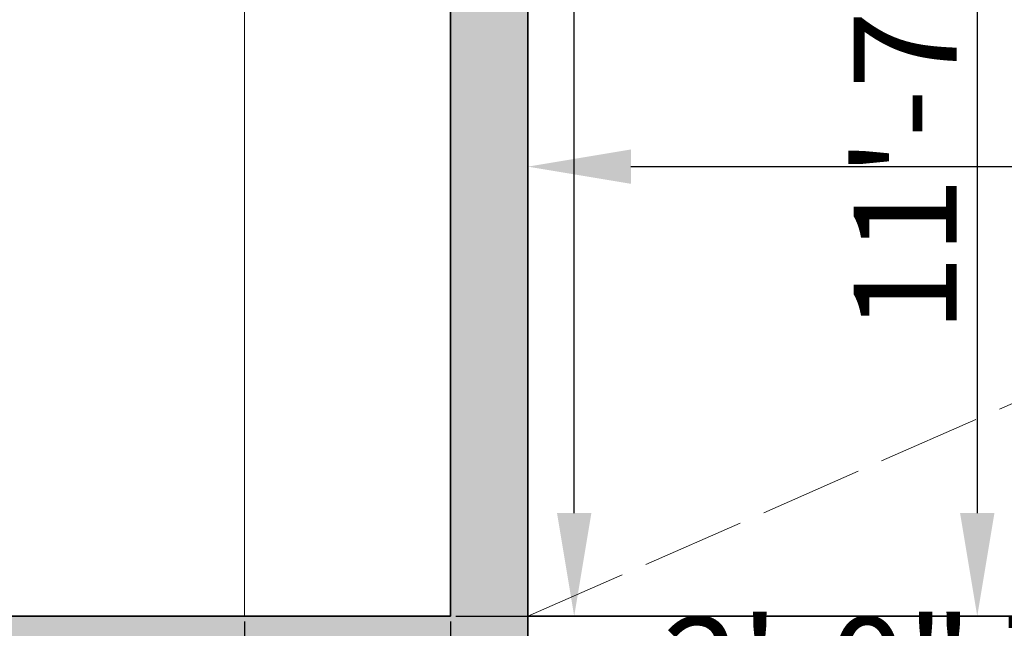
# Model space of a CAD drawing. Units: inches. Extents: x 2083 to 3317, y 1141 to 2115.
# Tile 86 of 256: x 2486 to 2600, y 1271 to 1342. Entities that reach past the tile are written whole.
import ezdxf

# ---------------------------------------------------------------- set-up
doc = ezdxf.new("R2010")
doc.units = ezdxf.units.IN
doc.linetypes.add('ACAD_ISO02W100', pattern=[15, 12, -3])
for name, color, linetype, lineweight in [('A-ANNO-DIMS', 2, 'Continuous', 18), ('A-FLOR-CASE', 8, 'Continuous', 18), ('A-FLOR-OPEN', 8, 'ACAD_ISO02W100', 13), ('A-WALL', 7, 'Continuous', 35)]:
    doc.layers.add(name, color=color, linetype=linetype, lineweight=lineweight)
doc.layers.add('A-WALL-PATT', color=251, linetype='Continuous', lineweight=13, true_color=0x636466)
doc.styles.get("Standard").update_dxf_attribs({"font": 'arial.ttf'})
doc.dimstyles.new('ISO-25', dxfattribs={"dimtxt": 12, "dimasz": 12, "dimexe": 1.25, "dimexo": 0.625, "dimtad": 1, "dimlunit": 3, "dimtxsty": 'Standard', "dimcen": 2.5, "dimadec": 0, "dimazin": 0, "dimtfac": 1, "dimtmove": 0, "dimatfit": 3, "dimfxl": 1, "dimarcsym": 0})

# ---------------------------------------------------------------- blocks, each defined once
blk = doc.blocks.new('CASEWORK-96X24')
for q in [(0, 0), (24, 96)]:
    blk.add_line((0, 96), q)
blk = doc.blocks.new('*D24')
at = {"layer": 'A-ANNO-DIMS', "color": 0, "lineweight": -2, "transparency": 16777216}
for p, q in [((2550.36, 1368.26), (2550.36, 1556.98)), ((2536.58, 1368.26), (2551.61, 1368.26)), ((2550.36, 1284.26), (2550.36, 1356.26)), ((2536.58, 1272.26), (2551.61, 1272.26))]:
    blk.add_line(p, q, dxfattribs=at)
at = {"layer": 'A-ANNO-DIMS', "color": 0, "transparency": 16777216}
for points in [[(2548.36, 1356.26), (2552.36, 1356.26), (2550.36, 1368.26)], [(2548.36, 1284.26), (2552.36, 1284.26), (2550.36, 1272.26)]]:
    blk.add_solid(points, dxfattribs=at)
at = {"layer": 'Defpoints', "color": 0, "transparency": 16777216}
for p in [(2535.96, 1368.26), (2550.36, 1368.26), (2535.96, 1272.26)]:
    blk.add_point(p, dxfattribs=at)
at = {"layer": 'A-ANNO-DIMS', "color": 0, "transparency": 16777216, "insert": (2543.53, 1468.62), "char_height": 12, "attachment_point": 5, "rotation": 90}
blk.add_mtext('CASEWORK 8\'-0" TYP.', dxfattribs=at)
blk = doc.blocks.new('*D25')
at = {"layer": 'A-ANNO-DIMS', "color": 0, "lineweight": -2, "transparency": 16777216}
for p, q in [((2511.96, 1271.64), (2511.96, 1256.61)), ((2535.96, 1271.64), (2535.96, 1256.61)), ((2499.96, 1257.86), (2487.96, 1257.86)), ((2511.96, 1257.86), (2535.96, 1257.86)), ((2547.96, 1257.86), (2634.56, 1257.86))]:
    blk.add_line(p, q, dxfattribs=at)
at = {"layer": 'A-ANNO-DIMS', "color": 0, "transparency": 16777216}
for points in [[(2499.96, 1259.86), (2499.96, 1255.86), (2511.96, 1257.86)], [(2547.96, 1259.86), (2547.96, 1255.86), (2535.96, 1257.86)]]:
    blk.add_solid(points, dxfattribs=at)
at = {"layer": 'Defpoints', "color": 0, "transparency": 16777216}
for p in [(2511.96, 1272.26), (2535.96, 1272.26), (2535.96, 1257.86)]:
    blk.add_point(p, dxfattribs=at)
at = {"layer": 'A-ANNO-DIMS', "color": 0, "transparency": 16777216, "insert": (2597.26, 1264.61), "char_height": 12, "attachment_point": 5}
blk.add_mtext('2\'-0" TYP.', dxfattribs=at)
blk = doc.blocks.new('*D66')
at = {"layer": 'A-ANNO-DIMS', "color": 0, "lineweight": -2, "transparency": 16777216}
for p, q in [((2544.96, 1272.89), (2544.96, 1325.86)), ((2862.96, 1272.89), (2862.96, 1325.86)), ((2556.96, 1324.61), (2850.96, 1324.61))]:
    blk.add_line(p, q, dxfattribs=at)
at = {"layer": 'A-ANNO-DIMS', "color": 0, "transparency": 16777216}
for points in [[(2556.96, 1326.61), (2556.96, 1322.61), (2544.96, 1324.61)], [(2850.96, 1326.61), (2850.96, 1322.61), (2862.96, 1324.61)]]:
    blk.add_solid(points, dxfattribs=at)
at = {"layer": 'Defpoints', "color": 0, "transparency": 16777216}
for p in [(2862.96, 1324.61), (2544.96, 1272.26), (2862.96, 1272.26)]:
    blk.add_point(p, dxfattribs=at)
at = {"layer": 'A-ANNO-DIMS', "color": 0, "transparency": 16777216, "insert": (2703.96, 1331.36), "char_height": 12, "attachment_point": 5}
blk.add_mtext('26\'-6"', dxfattribs=at)
blk = doc.blocks.new('*D67')
at = {"layer": 'A-ANNO-DIMS', "color": 0, "lineweight": -2, "transparency": 16777216}
for p, q in [((2545.58, 1411.76), (2598.56, 1411.76)), ((2597.31, 1399.76), (2597.31, 1284.26)), ((2545.58, 1272.26), (2598.56, 1272.26))]:
    blk.add_line(p, q, dxfattribs=at)
at = {"layer": 'A-ANNO-DIMS', "color": 0, "transparency": 16777216}
for points in [[(2595.31, 1399.76), (2599.31, 1399.76), (2597.31, 1411.76)], [(2595.31, 1284.26), (2599.31, 1284.26), (2597.31, 1272.26)]]:
    blk.add_solid(points, dxfattribs=at)
at = {"layer": 'Defpoints', "color": 0, "transparency": 16777216}
for p in [(2544.96, 1411.76), (2544.96, 1272.26), (2597.31, 1272.26)]:
    blk.add_point(p, dxfattribs=at)
at = {"layer": 'A-ANNO-DIMS', "color": 0, "transparency": 16777216, "insert": (2590.48, 1342.01), "char_height": 12, "attachment_point": 5, "rotation": 90}
blk.add_mtext('11\'-7 1/2"', dxfattribs=at)

msp = doc.modelspace()

# ---------------------------------------------------------------- hatches: boundary and pattern name
at = {"layer": 'A-WALL-PATT'}
h = msp.add_hatch(color=256, dxfattribs=at)
h.dxf.hatch_style = 1
h.paths.add_polyline_path([(3126.96, 2020.761), (2748.96, 2020.761), (2604.96, 2020.761), (2226.96, 2020.761), (2226.96, 1702.761), (2466.96, 1702.761), (2466.96, 1582.761), (2418.96, 1582.761), (2418.96, 1477.761), (2226.96, 1477.761), (2226.96, 1263.261), (2544.96, 1263.261), (2544.96, 1411.761), (2604.96, 1411.761), (2685.96, 1411.761), (2685.96, 1420.761), (2604.96, 1420.761), (2604.96, 1573.761), (2604.96, 1702.761), (2604.96, 2011.761), (2748.96, 2011.761), (2748.96, 1702.761), (2862.96, 1702.761), (2862.96, 1621.761), (2871.96, 1621.761), (2871.96, 1702.761), (2883.96, 1702.761), (2883.96, 1706.939, -0.0264593), (2883.96, 1711.761), (2757.96, 1711.761), (2757.96, 1807.761), (2787.96, 1807.761), (2787.96, 1812.261), (2757.96, 1812.261), (2757.96, 2011.761), (2877.96, 2011.761), (2877.96, 1812.261), (2847.96, 1812.261), (2847.96, 1807.761), (2889.836, 1807.761), (2889.836, 1812.261), (2882.46, 1812.261), (2882.46, 2011.761), (3117.96, 2011.761), (3117.96, 1812.261), (2937.836, 1812.261), (2937.836, 1807.761), (2995.71, 1807.761), (2995.71, 1796.118), (3000.21, 1796.118), (3000.21, 1807.761), (3117.96, 1807.761), (3117.96, 1711.761), (3000.21, 1711.761), (3000.21, 1760.118), (2998.573, 1760.118, -0.020711), (2995.71, 1760.118), (2995.71, 1711.761), (2931.96, 1711.761), (2931.96, 1702.761), (3126.96, 1702.761)])
h.paths.add_polyline_path([(2471.46, 2011.761), (2471.46, 1810.011), (2462.717, 1810.011), (2462.717, 1805.511), (2505.96, 1805.511), (2505.96, 1810.011), (2475.96, 1810.011), (2475.96, 2011.761), (2595.96, 2011.761), (2595.96, 1810.011), (2565.96, 1810.011), (2565.96, 1805.511), (2595.96, 1805.511), (2595.96, 1711.761), (2235.96, 1711.761), (2235.96, 1805.511), (2353.71, 1805.511), (2353.71, 1796.054), (2358.21, 1796.054), (2358.21, 1805.511), (2414.717, 1805.511), (2414.717, 1810.011), (2235.96, 1810.011), (2235.96, 2011.761)], flags=16)
h.paths.add_polyline_path([(2270.205, 1994.61), (2270.205, 1970.61), (2246.205, 1970.61), (2246.205, 1994.61)], flags=0)
edge = h.paths.add_edge_path(flags=0)
edge.add_ellipse((2332.027, 1899.798), major_axis=(-3.043, 3.043), ratio=0.1682525, start_angle=-161.33217, end_angle=-156.30711, ccw=False)
edge.add_ellipse((2333.082, 1898.744), major_axis=(-1.055, 1.055), ratio=0.4535321, start_angle=-123.37102, end_angle=-94.15911)
edge = h.paths.add_edge_path(flags=0)
edge.add_ellipse((2332.027, 1968.876), major_axis=(3.043, 3.043), ratio=0.1682525, start_angle=18.66783, end_angle=23.69289)
edge.add_spline(control_points=[(2332.926, 1970.691), (2332.227, 1970.336), (2330.894, 1969.659), (2328.413, 1970.932), (2327.204, 1967.749), (2324.71, 1969.956), (2322.533, 1967.012), (2320.013, 1971.296), (2317.68, 1968.158), (2316.041, 1967.102), (2315.427, 1966.81)], knot_values=[0, 0, 0, 0, 2.2670587, 4.3245589, 6.6855835, 8.8786411, 11.121502, 14.300359, 17.7552837, 19.732645, 19.732645, 19.732645, 19.732645], degree=3, periodic=0)
edge.add_ellipse((2332.027, 1968.876), major_axis=(3.043, 3.043), ratio=0.1682525, start_angle=18.66783, end_angle=23.69289, ccw=False)
edge.add_ellipse((2333.082, 1969.931), major_axis=(1.055, 1.055), ratio=0.4535321, start_angle=56.62898, end_angle=85.84089, ccw=False)
edge = h.paths.add_edge_path(flags=0)
edge.add_spline(control_points=[(2296.428, 1967.988), (2293.628, 1965.336), (2287.704, 1959.727), (2299.744, 1949.996), (2294.533, 1935.669), (2290.573, 1920.604), (2293.394, 1909.974), (2296.185, 1904.967)], knot_values=[0.0991853, 0.0991853, 0.0991853, 0.0991853, 0.3453009, 0.6198217, 0.9826526, 1.3860932, 1.8105546, 1.8105546, 1.8105546, 1.8105546], degree=3, periodic=0)
edge.add_spline(control_points=[(2296.185, 1904.967), (2297.384, 1902.619), (2298.001, 1901.949), (2298.553, 1901.468)], knot_values=[0.0062457, 0.0062457, 0.0062457, 0.0062457, 0.0554759, 0.0554759, 0.0554759, 0.0554759], degree=3, periodic=0)
edge.add_spline(control_points=[(2298.553, 1901.468), (2297.259, 1900.923), (2295.225, 1900.232), (2293.06, 1900.614), (2292.101, 1900.788), (2292.09, 1900.791)], knot_values=[0.3128349, 0.3128349, 0.3128349, 0.3128349, 0.4017797, 0.4749867, 0.4759027, 0.4759027, 0.4759027, 0.4759027], degree=3, periodic=0)
edge.add_arc((2292.794, 1904.664), 3.937, 215.4209, 259.69818, ccw=False)
edge.add_spline(control_points=[(2289.585, 1902.382), (2289.477, 1902.535), (2289.368, 1902.688), (2289.261, 1902.841)], knot_values=[0.1028719, 0.1028719, 0.1028719, 0.1028719, 0.1168958, 0.1168958, 0.1168958, 0.1168958], degree=3, periodic=0)
edge.add_spline(control_points=[(2289.261, 1902.841), (2288.687, 1902.55), (2287.64, 1902.02), (2285.881, 1901.874), (2283.853, 1901.504), (2281.72, 1899.711), (2278.467, 1899.493), (2276.157, 1901.883), (2272.259, 1899.804), (2267.778, 1901.843), (2262.244, 1900.184), (2257.415, 1901.782), (2254.318, 1900.726), (2253.178, 1900.337)], knot_values=[0, 0, 0, 0, 1.9079767, 3.4771759, 5.261074, 7.9728515, 11.6802485, 13.7179214, 16.9395917, 22.789562, 27.5025027, 33.5952153, 37.1456181, 37.1456181, 37.1456181, 37.1456181], degree=3, periodic=0)
edge.add_line((2253.178, 1900.337), (2250.244, 1902.841))
edge.add_line((2250.244, 1902.841), (2250.244, 1965.833))
edge.add_line((2250.244, 1965.833), (2253.178, 1968.337))
edge.add_spline(control_points=[(2253.178, 1968.337), (2254.318, 1967.948), (2257.415, 1966.892), (2262.244, 1968.49), (2267.778, 1966.831), (2271.527, 1968.537), (2273.876, 1967.828), (2274.207, 1967.728)], knot_values=[0, 0, 0, 0, 0.0901802, 0.2449351, 0.3646438, 0.5132331, 0.5378548, 0.5378548, 0.5378548, 0.5378548], degree=3, periodic=0)
edge.add_arc((2274.353, 1963.793), 3.937, 72.05113, 92.12795, ccw=False)
edge.add_arc((2281.297, 1985.23), 18.596, 252.05113, 288.56572)
edge.add_arc((2292.317, 1956.029), 12.646, 71.02679, 113.77822, ccw=False)
edge = h.paths.add_edge_path(flags=0)
edge.add_spline(control_points=[(2274.899, 1951.856), (2275.066, 1951.617), (2275.233, 1951.377), (2275.398, 1951.136)], knot_values=[1.4099157, 1.4099157, 1.4099157, 1.4099157, 1.4315903, 1.4315903, 1.4315903, 1.4315903], degree=3, periodic=0)
edge.add_spline(control_points=[(2275.398, 1951.136), (2275.792, 1950.562), (2276.179, 1949.984), (2276.546, 1949.397)], knot_values=[1.3582378, 1.3582378, 1.3582378, 1.3582378, 1.4099157, 1.4099157, 1.4099157, 1.4099157], degree=3, periodic=0)
edge.add_line((2276.546, 1949.397), (2277.437, 1947.862))
edge.add_spline(control_points=[(2277.437, 1947.862), (2276.304, 1945.673), (2274.64, 1942.427), (2274.632, 1938.094), (2272.799, 1930.852), (2274.356, 1943.897), (2275.948, 1947.923), (2276.546, 1949.397)], knot_values=[0.0056315, 0.0056315, 0.0056315, 0.0056315, 0.1860139, 0.2660015, 0.3570872, 0.5963902, 0.7397317, 0.7397317, 0.7397317, 0.7397317], degree=3, periodic=0)
edge.add_spline(control_points=[(2276.546, 1949.397), (2276.179, 1949.984), (2275.792, 1950.562), (2275.398, 1951.136)], knot_values=[1.3582378, 1.3582378, 1.3582378, 1.3582378, 1.4099157, 1.4099157, 1.4099157, 1.4099157], degree=3, periodic=0)
edge.add_spline(control_points=[(2275.398, 1951.136), (2274.943, 1950.08), (2274.208, 1948.025), (2273.935, 1944.851), (2272.469, 1937.627), (2273.466, 1945.696), (2274.701, 1951.059), (2274.899, 1951.856)], knot_values=[0.1043639, 0.1043639, 0.1043639, 0.1043639, 0.1896363, 0.2696239, 0.3607096, 0.6000126, 0.6446217, 0.6446217, 0.6446217, 0.6446217], degree=3, periodic=0)
h.paths.add_polyline_path([(2269.168, 1963.128, -0.3575267), (2268.171, 1960.976, -0.0925607), (2268.171, 1939.436, -0.3575267), (2269.168, 1937.285, -0.3575267), (2267.016, 1938.282, -0.1647847), (2254.686, 1938.282, -0.3575267), (2252.534, 1937.285, -0.3575267), (2253.531, 1939.436, -0.0925607), (2253.531, 1960.976, -0.3575267), (2252.534, 1963.128, -0.3575267), (2254.686, 1962.131, -0.1647847), (2267.016, 1962.131, -0.3575267)], flags=0)
h.paths.add_polyline_path([(2248.874, 1967.802), (2248.874, 1957.028), (2249.458, 1957.028), (2249.458, 1911.647), (2248.874, 1911.647), (2248.874, 1900.873), (2246.512, 1900.873, 0.1973271), (2244.15, 1902.457), (2244.15, 1966.218, 0.1973271), (2246.512, 1967.802)], flags=0)
h.paths.add_polyline_path([(2269.168, 1931.389, -0.3575267), (2268.171, 1929.238, -0.0925607), (2268.171, 1907.698, -0.3575267), (2269.168, 1905.547, -0.3575267), (2267.016, 1906.544, -0.1647847), (2254.686, 1906.544, -0.3575267), (2252.534, 1905.547, -0.3575267), (2253.531, 1907.698, -0.0925607), (2253.531, 1929.238, -0.3575267), (2252.534, 1931.389, -0.3575267), (2254.686, 1930.392, -0.1647847), (2267.016, 1930.392, -0.3575267)], flags=0)
edge = h.paths.add_edge_path(flags=0)
edge.add_spline(control_points=[(2276.197, 1906.724), (2276.168, 1909.029), (2276.114, 1913.372), (2270.598, 1924.925), (2273.905, 1919.013), (2275.922, 1916.262), (2275.475, 1912.402), (2277.258, 1910.381), (2276.696, 1908.225), (2276.646, 1906.813), (2276.618, 1906.008)], knot_values=[0, 0, 0, 0, 8.6102597, 16.2212739, 18.8430575, 23.8048978, 27.4408283, 29.3561016, 31.2034776, 33.6506866, 33.6506866, 33.6506866, 33.6506866], degree=3, periodic=0)
edge.add_spline(control_points=[(2276.618, 1906.008), (2276.623, 1905.624), (2276.498, 1904.629), (2275.442, 1903.855), (2274.937, 1903.08), (2274.859, 1902.841)], knot_values=[0.1564884, 0.1564884, 0.1564884, 0.1564884, 0.1843975, 0.2313765, 0.2505985, 0.2505985, 0.2505985, 0.2505985], degree=3, periodic=0)
edge.add_line((2274.859, 1902.841), (2276.506, 1902.841))
edge.add_spline(control_points=[(2276.506, 1902.841), (2276.788, 1903.085), (2277.665, 1904.125), (2278.25, 1904.341), (2277.654, 1908.527), (2278.156, 1906.228), (2278.1, 1905.286), (2278.847, 1904.069), (2277.857, 1903.415), (2277.874, 1902.991), (2277.904, 1902.841)], knot_values=[0.0595743, 0.0595743, 0.0595743, 0.0595743, 0.0807529, 0.1037415, 0.1697201, 0.1760361, 0.2071372, 0.2404744, 0.2623409, 0.2736605, 0.2736605, 0.2736605, 0.2736605], degree=3, periodic=0)
edge.add_line((2277.904, 1902.841), (2280.03, 1902.841))
edge.add_spline(control_points=[(2280.03, 1902.841), (2279.888, 1903.088), (2279.499, 1903.982), (2280.152, 1905.939), (2278.104, 1909.658), (2279.762, 1907.185), (2280.328, 1904.875), (2280.485, 1903.49), (2281.463, 1903.249), (2281.758, 1902.936), (2281.834, 1902.841)], knot_values=[0.013856, 0.013856, 0.013856, 0.013856, 0.0348738, 0.0888667, 0.1078792, 0.1267378, 0.158714, 0.1937575, 0.2174868, 0.2267221, 0.2267221, 0.2267221, 0.2267221], degree=3, periodic=0)
edge.add_spline(control_points=[(2281.834, 1902.841), (2281.788, 1902.827), (2281.647, 1902.783), (2281.396, 1902.859), (2281.088, 1902.985), (2280.721, 1903.061), (2280.333, 1903.026), (2280.125, 1902.899), (2280.03, 1902.841)], knot_values=[0, 0, 0, 0, 0.1441304, 0.435517, 0.7492759, 1.1530457, 1.5483707, 1.878348, 1.878348, 1.878348, 1.878348], degree=3, periodic=0)
edge.add_line((2280.03, 1902.841), (2277.904, 1902.841))
edge.add_spline(control_points=[(2277.904, 1902.841), (2277.893, 1902.796), (2277.865, 1902.68), (2277.607, 1902.687), (2277.274, 1902.801), (2276.838, 1902.62), (2276.584, 1902.789), (2276.506, 1902.841)], knot_values=[0, 0, 0, 0, 0.1271885, 0.3261988, 0.6280094, 1.2435704, 1.5153306, 1.5153306, 1.5153306, 1.5153306], degree=3, periodic=0)
edge.add_line((2276.506, 1902.841), (2274.859, 1902.841))
edge.add_spline(control_points=[(2274.859, 1902.841), (2274.814, 1902.899), (2274.725, 1903.013), (2274.493, 1903.119), (2274.244, 1902.961), (2273.937, 1903.185), (2273.614, 1902.983), (2273.408, 1902.883), (2273.322, 1902.841)], knot_values=[0, 0, 0, 0, 0.2184302, 0.4369566, 0.6879766, 0.9903786, 1.3983955, 1.6918498, 1.6918498, 1.6918498, 1.6918498], degree=3, periodic=0)
edge.add_spline(control_points=[(2273.322, 1902.841), (2273.617, 1903.446), (2274.274, 1904.538), (2276.027, 1904.574), (2276.207, 1906.584), (2276.197, 1906.724)], knot_values=[0.0122268, 0.0122268, 0.0122268, 0.0122268, 0.0594721, 0.1062177, 0.134458, 0.134458, 0.134458, 0.134458], degree=3, periodic=0)
h.paths.add_polyline_path([(2270.776, 1897.79), (2270.776, 1873.79), (2246.776, 1873.79), (2246.776, 1897.79)], flags=0)
h.paths.add_polyline_path([(2353.71, 1760.005), (2353.71, 1760.054), (2358.21, 1760.054, -0.033729)], flags=0)
h.paths.add_polyline_path([(2321.819, 1737.529), (2341.995, 1737.529, -0.4142136), (2343.203, 1736.321), (2343.203, 1721.021, -0.4142136), (2341.995, 1719.813), (2321.819, 1719.813, -0.4142136), (2320.611, 1721.021), (2320.611, 1736.321, -0.4142136)], flags=0)
h.paths.add_polyline_path([(2324.235, 1736.321), (2339.579, 1736.321, -0.4142136), (2341.995, 1733.905), (2341.995, 1725.45, -0.4142136), (2339.579, 1723.034), (2333.681, 1723.034), (2333.845, 1722.045, -0.8706461), (2335.425, 1721.826, -0.767327), (2333.923, 1721.423), (2331.291, 1721.423, -0.767327), (2329.788, 1721.826, -0.8706461), (2331.368, 1722.045), (2331.533, 1723.034), (2324.235, 1723.034, -0.4142136), (2321.819, 1725.45), (2321.819, 1733.905, -0.4142136)], flags=0)
h.paths.add_polyline_path([(2570.484, 1928.615), (2589.684, 1928.615), (2590.169, 1928.615), (2590.169, 1904.993), (2570.484, 1904.993)], flags=0)
h.paths.add_polyline_path([(2574.447, 1927.264, -1), (2572.829, 1927.264, -1)], flags=0)
h.paths.add_polyline_path([(2573.09, 1926.941), (2573.925, 1927.776), (2574.148, 1927.553), (2573.313, 1926.718)], flags=0)
h.paths.add_polyline_path([(2578.779, 1919.73, -1), (2571.592, 1919.73, -1)], flags=0)
h.paths.add_polyline_path([(2578.385, 1919.73, -1), (2571.985, 1919.73, -1)], flags=0)
h.paths.add_polyline_path([(2331.596, 1729.476, -1), (2333.618, 1729.476, -1)], flags=0)
h.paths.add_polyline_path([(2578.034, 1927.264, -1), (2576.416, 1927.264, -1)], flags=0)
h.paths.add_polyline_path([(2576.689, 1927.531), (2576.912, 1927.754), (2577.747, 1926.919), (2577.524, 1926.696)], flags=0)
h.paths.add_polyline_path([(2578.139, 1909.86, -1), (2572.232, 1909.86, -1)], flags=0)
h.paths.add_polyline_path([(2577.745, 1909.86, -1), (2572.625, 1909.86, -1)], flags=0)
h.paths.add_polyline_path([(2583.798, 1927.264, -1), (2582.179, 1927.264, -1)], flags=0)
h.paths.add_polyline_path([(2582.719, 1927.754), (2583.554, 1926.919), (2583.331, 1926.696), (2582.496, 1927.531)], flags=0)
h.paths.add_polyline_path([(2582.496, 1927.531), (2582.719, 1927.754), (2583.554, 1926.919), (2583.331, 1926.696)], flags=0)
h.paths.add_polyline_path([(2587.739, 1920.53, -1), (2581.832, 1920.53, -1)], flags=0)
h.paths.add_polyline_path([(2587.345, 1920.53, -1), (2582.225, 1920.53, -1)], flags=0)
h.paths.add_polyline_path([(2587.385, 1927.264, -1), (2585.766, 1927.264, -1)], flags=0)
h.paths.add_polyline_path([(2586.082, 1926.98), (2586.917, 1927.815), (2587.14, 1927.593), (2586.305, 1926.758)], flags=0)
h.paths.add_polyline_path([(2588.379, 1910.66, -1), (2581.192, 1910.66, -1)], flags=0)
h.paths.add_polyline_path([(2587.985, 1910.66, -1), (2581.585, 1910.66, -1)], flags=0)
h.paths.add_polyline_path([(2417.168, 1729.478), (2437.344, 1729.478, -0.4142136), (2438.552, 1728.27), (2438.552, 1712.969, -0.4142136), (2437.344, 1711.761), (2417.168, 1711.761, -0.4142136), (2415.96, 1712.969), (2415.96, 1728.27, -0.4142136)], flags=0)
h.paths.add_polyline_path([(2419.584, 1728.27), (2434.928, 1728.27, -0.4142136), (2437.344, 1725.854), (2437.344, 1717.398, -0.4142136), (2434.928, 1714.983), (2429.029, 1714.983), (2429.194, 1713.994, -0.8706461), (2430.774, 1713.775, -0.767327), (2429.271, 1713.372), (2426.64, 1713.372, -0.767327), (2425.137, 1713.775, -0.8706461), (2426.717, 1713.994), (2426.882, 1714.983), (2419.584, 1714.983, -0.4142136), (2417.168, 1717.398), (2417.168, 1725.854, -0.4142136)], flags=0)
h.paths.add_polyline_path([(2419.584, 1728.27), (2434.928, 1728.27, -0.4142136), (2437.344, 1725.854), (2437.344, 1717.398, -0.4142136), (2434.928, 1714.983), (2429.029, 1714.983), (2428.358, 1719.009), (2427.553, 1719.009), (2426.882, 1714.983), (2419.584, 1714.983, -0.4142136), (2417.168, 1717.398), (2417.168, 1725.854, -0.4142136)], flags=0)
h.paths.add_polyline_path([(2426.944, 1721.425, -1), (2428.967, 1721.425, -1)], flags=0)
h.paths.add_polyline_path([(2475.96, 1702.761), (2595.96, 1702.761), (2595.96, 1582.761), (2475.96, 1582.761)], flags=16)
h.paths.add_polyline_path([(2427.96, 1573.761), (2595.96, 1573.761), (2595.96, 1468.761), (2595.96, 1420.761), (2384.46, 1420.761), (2384.46, 1468.761), (2427.96, 1468.761)], flags=16)
h.paths.add_polyline_path([(2379.96, 1468.761), (2379.96, 1420.761), (2235.96, 1420.761), (2235.96, 1468.761)], flags=16)
h.paths.add_polyline_path([(2317.816, 1466.696), (2337.992, 1466.696, -0.4142136), (2339.2, 1465.488), (2339.2, 1450.187, -0.4142136), (2337.992, 1448.979), (2317.816, 1448.979, -0.4142136), (2316.608, 1450.187), (2316.608, 1465.488, -0.4142136)], flags=0)
h.paths.add_polyline_path([(2320.232, 1465.488), (2335.576, 1465.488, -0.4142136), (2337.992, 1463.072), (2337.992, 1454.616, -0.4142136), (2335.576, 1452.2), (2329.677, 1452.2), (2329.842, 1451.212, -0.8706461), (2331.422, 1450.992, -0.767327), (2329.92, 1450.59), (2327.288, 1450.59, -0.767327), (2325.785, 1450.992, -0.8706461), (2327.365, 1451.212), (2327.53, 1452.2), (2320.232, 1452.2, -0.4142136), (2317.816, 1454.616), (2317.816, 1463.072, -0.4142136)], flags=0)
h.paths.add_polyline_path([(2320.232, 1465.488), (2335.576, 1465.488, -0.4142136), (2337.992, 1463.072), (2337.992, 1454.616, -0.4142136), (2335.576, 1452.2), (2329.677, 1452.2), (2329.006, 1456.227), (2328.201, 1456.227), (2327.53, 1452.2), (2320.232, 1452.2, -0.4142136), (2317.816, 1454.616), (2317.816, 1463.072, -0.4142136)], flags=0)
h.paths.add_polyline_path([(2327.593, 1458.643, -1), (2329.615, 1458.643, -1)], flags=0)
h.paths.add_polyline_path([(2244.412, 1433.34), (2241.921, 1433.34, -0.4142136), (2240.018, 1435.244), (2240.018, 1440.953, -0.4142105), (2241.921, 1442.856), (2244.412, 1442.856, -1.9764724)], flags=0)
h.paths.add_polyline_path([(2245.357, 1434.398, -0.4142136), (2245.357, 1441.799, -2.1440985)], flags=0)
h.paths.add_polyline_path([(2535.96, 1416.261), (2535.96, 1272.261), (2235.96, 1272.261), (2235.96, 1416.261)], flags=16)
h.paths.add_polyline_path([(2260.12, 1384.293), (2260.12, 1362.039), (2237.865, 1362.039), (2237.865, 1384.293)], flags=0)
edge = h.paths.add_edge_path(flags=0)
edge.add_line((2318.252, 1362.093), (2318.146, 1362.001))
edge.add_ellipse((2317.445, 1360.431), major_axis=(2.822, 2.822), ratio=0.1682525, start_angle=18.66783, end_angle=20.94813, ccw=False)
edge.add_ellipse((2318.423, 1361.409), major_axis=(0.978, 0.978), ratio=0.4535321, start_angle=56.62898, end_angle=70.2262, ccw=False)
edge = h.paths.add_edge_path(flags=0)
edge.add_line((2319.107, 1295.571), (2319.015, 1295.677))
edge.add_ellipse((2317.445, 1296.378), major_axis=(-2.822, 2.822), ratio=0.1682525, start_angle=-161.33217, end_angle=-159.05187, ccw=False)
edge.add_ellipse((2318.423, 1295.4), major_axis=(-0.978, 0.978), ratio=0.4535321, start_angle=-123.37102, end_angle=-109.7738)
edge = h.paths.add_edge_path(flags=0)
edge.add_spline(control_points=[(2284.21, 1301.17), (2284.581, 1300.445), (2284.891, 1299.892), (2285.16, 1299.461)], knot_values=[0.0390658, 0.0390658, 0.0390658, 0.0390658, 0.0554759, 0.0554759, 0.0554759, 0.0554759], degree=3, periodic=0)
edge.add_line((2285.16, 1299.461), (2284.21, 1301.17))
edge = h.paths.add_edge_path(flags=0)
edge.add_line((2280.412, 1297.298), (2283.37, 1297.036))
edge.add_line((2283.37, 1297.036), (2286.406, 1297.926))
edge.add_spline(control_points=[(2286.406, 1297.926), (2285.305, 1297.463), (2284.345, 1297.129), (2283.37, 1297.036)], knot_values=[0.3943688, 0.3943688, 0.3943688, 0.3943688, 0.4759027, 0.4759027, 0.4759027, 0.4759027], degree=3, periodic=0)
edge.add_spline(control_points=[(2283.37, 1297.036), (2283.281, 1297.028), (2282.316, 1296.957), (2281.313, 1297.134), (2280.423, 1297.296), (2280.412, 1297.298)], knot_values=[0.3128349, 0.3128349, 0.3128349, 0.3128349, 0.3202458, 0.3934528, 0.3943688, 0.3943688, 0.3943688, 0.3943688], degree=3, periodic=0)
edge = h.paths.add_edge_path(flags=0)
edge.add_line((2284.436, 1359.607), (2280.446, 1355.328))
edge.add_line((2280.446, 1355.328), (2279.58, 1351.018))
edge.add_line((2279.58, 1351.018), (2282.413, 1346.58))
edge.add_spline(control_points=[(2282.413, 1346.58), (2283.153, 1345.589), (2284.253, 1344.029), (2284.801, 1342.387), (2284.935, 1341.806)], knot_values=[1.2400982, 1.2400982, 1.2400982, 1.2400982, 1.3328922, 1.3827123, 1.3827123, 1.3827123, 1.3827123], degree=3, periodic=0)
edge.add_spline(control_points=[(2284.935, 1341.806), (2285.319, 1340.141), (2285.233, 1338.409), (2284.91, 1336.654)], knot_values=[1.0974841, 1.0974841, 1.0974841, 1.0974841, 1.2400982, 1.2400982, 1.2400982, 1.2400982], degree=3, periodic=0)
edge.add_spline(control_points=[(2284.91, 1336.654), (2284.587, 1334.899), (2284.027, 1333.12), (2283.463, 1331.361)], knot_values=[0.9548699, 0.9548699, 0.9548699, 0.9548699, 1.0974841, 1.0974841, 1.0974841, 1.0974841], degree=3, periodic=0)
edge.add_line((2283.463, 1331.361), (2281.89, 1326.153))
edge.add_line((2281.89, 1326.153), (2280.756, 1321.056))
edge.add_line((2280.756, 1321.056), (2280.299, 1316.002))
edge.add_line((2280.299, 1316.002), (2280.716, 1310.95))
edge.add_line((2280.716, 1310.95), (2282.028, 1305.972))
edge.add_line((2282.028, 1305.972), (2284.21, 1301.17))
edge.add_spline(control_points=[(2284.21, 1301.17), (2283.341, 1302.73), (2282.612, 1304.336), (2282.028, 1305.972)], knot_values=[0.0991853, 0.0991853, 0.0991853, 0.0991853, 0.2417994, 0.2417994, 0.2417994, 0.2417994], degree=3, periodic=0)
edge.add_spline(control_points=[(2282.028, 1305.972), (2281.444, 1307.608), (2281.005, 1309.273), (2280.716, 1310.95)], knot_values=[0.2417994, 0.2417994, 0.2417994, 0.2417994, 0.3844135, 0.3844135, 0.3844135, 0.3844135], degree=3, periodic=0)
edge.add_spline(control_points=[(2280.716, 1310.95), (2280.433, 1312.588), (2280.289, 1314.277), (2280.299, 1315.962), (2280.299, 1316.002)], knot_values=[0.3844135, 0.3844135, 0.3844135, 0.3844135, 0.5236467, 0.5270276, 0.5270276, 0.5270276, 0.5270276], degree=3, periodic=0)
edge.add_spline(control_points=[(2280.299, 1316.002), (2280.312, 1317.687), (2280.478, 1319.368), (2280.756, 1321.056)], knot_values=[0.5270276, 0.5270276, 0.5270276, 0.5270276, 0.6696417, 0.6696417, 0.6696417, 0.6696417], degree=3, periodic=0)
edge.add_spline(control_points=[(2280.756, 1321.056), (2281.035, 1322.744), (2281.426, 1324.44), (2281.89, 1326.153)], knot_values=[0.6696417, 0.6696417, 0.6696417, 0.6696417, 0.8122558, 0.8122558, 0.8122558, 0.8122558], degree=3, periodic=0)
edge.add_spline(control_points=[(2281.89, 1326.153), (2282.264, 1327.533), (2282.788, 1329.262), (2283.353, 1331.018), (2283.463, 1331.361)], knot_values=[0.8122558, 0.8122558, 0.8122558, 0.8122558, 0.9270873, 0.9548699, 0.9548699, 0.9548699, 0.9548699], degree=3, periodic=0)
edge.add_line((2283.463, 1331.361), (2284.91, 1336.654))
edge.add_line((2284.91, 1336.654), (2284.935, 1341.806))
edge.add_line((2284.935, 1341.806), (2282.413, 1346.58))
edge.add_spline(control_points=[(2282.413, 1346.58), (2281.275, 1348.104), (2280.078, 1349.57), (2279.58, 1351.018)], knot_values=[1.3827123, 1.3827123, 1.3827123, 1.3827123, 1.5253264, 1.5253264, 1.5253264, 1.5253264], degree=3, periodic=0)
edge.add_spline(control_points=[(2279.58, 1351.018), (2279.443, 1351.415), (2279.136, 1352.857), (2279.735, 1354.29), (2280.446, 1355.328)], knot_values=[1.5253264, 1.5253264, 1.5253264, 1.5253264, 1.564439, 1.6679405, 1.6679405, 1.6679405, 1.6679405], degree=3, periodic=0)
edge.add_spline(control_points=[(2280.446, 1355.328), (2281.426, 1356.758), (2282.931, 1358.183), (2284.436, 1359.607)], knot_values=[1.6679405, 1.6679405, 1.6679405, 1.6679405, 1.8105546, 1.8105546, 1.8105546, 1.8105546], degree=3, periodic=0)
edge.add_arc((2280.623, 1348.518), 11.726, 71.02679, 113.77822)
edge.add_arc((2270.405, 1375.595), 17.244, 252.05113, 288.56572, ccw=False)
edge.add_arc((2263.966, 1355.718), 3.651, 72.05113, 92.12795)
edge.add_arc((2263.966, 1355.718), 3.651, 92.12795, 177.98513)
edge.add_spline(control_points=[(2260.318, 1355.846), (2260.26, 1354.221), (2260.551, 1350.187), (2262.999, 1346.766), (2264.473, 1344.649)], knot_values=[1.4315903, 1.4315903, 1.4315903, 1.4315903, 1.5641438, 1.7706953, 1.7706953, 1.7706953, 1.7706953], degree=3, periodic=0)
edge.add_line((2264.473, 1344.649), (2264.936, 1343.983))
edge.add_spline(control_points=[(2263.801, 1340.248), (2263.843, 1340.514), (2264.067, 1341.756), (2264.513, 1343.002), (2264.935, 1343.981)], knot_values=[0.5365702, 0.5365702, 0.5365702, 0.5365702, 0.5593494, 0.6446217, 0.6446217, 0.6446217, 0.6446217], degree=3, periodic=0)
edge.add_spline(control_points=[(2264.935, 1343.981), (2265.118, 1343.715), (2265.299, 1343.448), (2265.477, 1343.179)], knot_values=[1.3840767, 1.3840767, 1.3840767, 1.3840767, 1.4099157, 1.4099157, 1.4099157, 1.4099157], degree=3, periodic=0)
edge.add_spline(control_points=[(2265.477, 1343.179), (2265.655, 1342.911), (2265.829, 1342.641), (2265.999, 1342.369)], knot_values=[1.3582378, 1.3582378, 1.3582378, 1.3582378, 1.3840767, 1.3840767, 1.3840767, 1.3840767], degree=3, periodic=0)
edge.add_line((2265.999, 1342.369), (2266.826, 1340.946))
edge.add_spline(control_points=[(2266.826, 1340.946), (2268.894, 1337.09), (2271.398, 1325.843), (2270.516, 1310.569), (2275.919, 1301.861), (2277.79, 1299.199)], knot_values=[0.1168958, 0.1168958, 0.1168958, 0.1168958, 0.4729873, 1.0509689, 1.3137934, 1.3137934, 1.3137934, 1.3137934], degree=3, periodic=0)
edge.add_spline(control_points=[(2277.79, 1299.199), (2277.839, 1299.128), (2277.889, 1299.057), (2277.94, 1298.987)], knot_values=[0.1098839, 0.1098839, 0.1098839, 0.1098839, 0.1168958, 0.1168958, 0.1168958, 0.1168958], degree=3, periodic=0)
edge.add_line((2277.94, 1298.987), (2277.789, 1299.199))
edge.add_spline(control_points=[(2277.789, 1299.199), (2277.257, 1298.929), (2276.286, 1298.438), (2275.039, 1298.334), (2274.383, 1298.239), (2274.215, 1298.209)], knot_values=[33.1218702, 33.1218702, 33.1218702, 33.1218702, 35.0290557, 36.5982549, 37.1448269, 37.1448269, 37.1448269, 37.1448269], degree=3, periodic=0)
edge.add_line((2274.215, 1298.209), (2273.073, 1297.893))
edge.add_spline(control_points=[(2273.073, 1297.893), (2272.323, 1297.58), (2271.039, 1296.511), (2269.248, 1296.226), (2268.423, 1296.375)], knot_values=[26.5325843, 26.5325843, 26.5325843, 26.5325843, 29.198919, 31.8391012, 31.8391012, 31.8391012, 31.8391012], degree=3, periodic=0)
edge.add_line((2268.423, 1296.375), (2263.879, 1297.458))
edge.add_spline(control_points=[(2263.879, 1297.458), (2263.556, 1297.359), (2261.86, 1296.839), (2260.239, 1297.282), (2258.933, 1297.516)], knot_values=[15.9195506, 15.9195506, 15.9195506, 15.9195506, 16.9395917, 21.2260675, 21.2260675, 21.2260675, 21.2260675], degree=3, periodic=0)
edge.add_line((2258.933, 1297.516), (2254.055, 1297.329))
edge.add_spline(control_points=[(2254.055, 1297.329), (2253.756, 1297.296), (2252.114, 1297.165), (2250.462, 1297.544), (2249.13, 1297.668)], knot_values=[5.3065169, 5.3065169, 5.3065169, 5.3065169, 6.2764352, 10.6130337, 10.6130337, 10.6130337, 10.6130337], degree=3, periodic=0)
edge.add_line((2249.13, 1297.668), (2244.332, 1296.878))
edge.add_line((2244.332, 1296.878), (2241.611, 1299.199))
edge.add_line((2241.611, 1299.199), (2241.611, 1357.609))
edge.add_line((2241.611, 1357.609), (2244.332, 1359.931))
edge.add_line((2244.332, 1359.931), (2252.729, 1359.543))
edge.add_spline(control_points=[(2252.729, 1359.543), (2252.871, 1359.546), (2253.306, 1359.548), (2253.74, 1359.514), (2254.032, 1359.482)], knot_values=[0.233291, 0.233291, 0.233291, 0.233291, 0.2449351, 0.2689274, 0.2689274, 0.2689274, 0.2689274], degree=3, periodic=0)
edge.add_line((2254.032, 1359.482), (2259.587, 1359.416))
edge.add_spline(control_points=[(2259.587, 1359.416), (2260.677, 1359.629), (2262.073, 1359.897), (2263.524, 1359.459), (2263.83, 1359.366)], knot_values=[0.4225164, 0.4225164, 0.4225164, 0.4225164, 0.5132331, 0.5378548, 0.5378548, 0.5378548, 0.5378548], degree=3, periodic=0)
edge.add_arc((2263.966, 1355.718), 3.651, 72.05113, 92.12795, ccw=False)
edge.add_arc((2270.405, 1375.595), 17.244, 252.05113, 288.56572)
edge.add_arc((2280.623, 1348.518), 11.726, 71.02679, 113.77822, ccw=False)
h.paths.add_polyline_path([(2240.341, 1359.435), (2240.341, 1349.444), (2240.882, 1349.444), (2240.882, 1307.365), (2240.341, 1307.365), (2240.341, 1297.374), (2238.15, 1297.374, 0.1973271), (2235.96, 1298.843), (2235.96, 1357.966, 0.1973271), (2238.15, 1359.435)], flags=0)
h.paths.add_polyline_path([(2259.158, 1355.101, -0.3575267), (2258.233, 1353.106, -0.0925607), (2258.233, 1333.133, -0.3575267), (2259.158, 1331.138, -0.3575267), (2257.163, 1332.062, -0.1647847), (2245.729, 1332.062, -0.3575267), (2243.735, 1331.138, -0.3575267), (2244.659, 1333.133, -0.0925607), (2244.659, 1353.106, -0.3575267), (2243.735, 1355.101, -0.3575267), (2245.729, 1354.176, -0.1647847), (2257.163, 1354.176, -0.3575267)], flags=0)
edge = h.paths.add_edge_path(flags=0)
edge.add_line((2265.999, 1342.369), (2266.826, 1340.946))
edge.add_line((2266.826, 1340.946), (2265.308, 1337.814))
edge.add_line((2265.308, 1337.814), (2264.358, 1334.653))
edge.add_line((2264.358, 1334.653), (2264.262, 1333.8))
edge.add_spline(control_points=[(2264.262, 1333.8), (2264.208, 1333.187), (2264.162, 1332.366), (2264.007, 1331.414), (2263.969, 1331.202)], knot_values=[0.4644442, 0.4644442, 0.4644442, 0.4644442, 0.5166905, 0.5316081, 0.5316081, 0.5316081, 0.5316081], degree=3, periodic=0)
edge.add_spline(control_points=[(2263.969, 1331.202), (2263.775, 1330.119), (2263.424, 1328.791), (2263.257, 1328.531), (2263.234, 1328.515)], knot_values=[0.3726816, 0.3726816, 0.3726816, 0.3726816, 0.4488497, 0.4644442, 0.4644442, 0.4644442, 0.4644442], degree=3, periodic=0)
edge.add_spline(control_points=[(2263.234, 1328.515), (2263.096, 1328.42), (2263.131, 1329.301), (2263.275, 1330.616)], knot_values=[0.2809191, 0.2809191, 0.2809191, 0.2809191, 0.3726816, 0.3726816, 0.3726816, 0.3726816], degree=3, periodic=0)
edge.add_spline(control_points=[(2263.275, 1330.616), (2263.419, 1331.93), (2263.672, 1333.677), (2263.97, 1335.315)], knot_values=[0.1891566, 0.1891566, 0.1891566, 0.1891566, 0.2809191, 0.2809191, 0.2809191, 0.2809191], degree=3, periodic=0)
edge.add_spline(control_points=[(2263.97, 1335.315), (2264.1, 1336.032), (2264.419, 1337.622), (2264.755, 1338.864), (2264.947, 1339.491)], knot_values=[0.097394, 0.097394, 0.097394, 0.097394, 0.1375775, 0.1891566, 0.1891566, 0.1891566, 0.1891566], degree=3, periodic=0)
edge.add_spline(control_points=[(2264.947, 1339.491), (2265.29, 1340.606), (2265.644, 1341.494), (2265.999, 1342.369)], knot_values=[0.0056315, 0.0056315, 0.0056315, 0.0056315, 0.097394, 0.097394, 0.097394, 0.097394], degree=3, periodic=0)
h.paths.add_polyline_path([(2259.158, 1325.671, -0.3575267), (2258.233, 1323.676, -0.0925607), (2258.233, 1303.703, -0.3575267), (2259.158, 1301.708, -0.3575267), (2257.163, 1302.633, -0.1647847), (2245.729, 1302.633, -0.3575267), (2243.735, 1301.708, -0.3575267), (2244.659, 1303.703, -0.0925607), (2244.659, 1323.676, -0.3575267), (2243.735, 1325.671, -0.3575267), (2245.729, 1324.747, -0.1647847), (2257.163, 1324.747, -0.3575267)], flags=0)
edge = h.paths.add_edge_path(flags=0)
edge.add_spline(control_points=[(2261.709, 1317.311), (2261.679, 1317.418), (2261.762, 1317.389), (2262.491, 1316.09), (2262.962, 1315.301)], knot_values=[14.9558607, 14.9558607, 14.9558607, 14.9558607, 16.2212739, 18.6948259, 18.6948259, 18.6948259, 18.6948259], degree=3, periodic=0)
edge.add_spline(control_points=[(2262.962, 1315.301), (2262.99, 1315.254), (2263.702, 1314.067), (2264.349, 1313.127), (2264.73, 1312.164)], knot_values=[18.6948259, 18.6948259, 18.6948259, 18.6948259, 18.8430575, 22.433791, 22.433791, 22.433791, 22.433791], degree=3, periodic=0)
edge.add_spline(control_points=[(2264.73, 1312.164), (2264.876, 1311.796), (2265.177, 1310.77), (2265.143, 1309.559), (2265.248, 1308.824)], knot_values=[22.433791, 22.433791, 22.433791, 22.433791, 23.8048978, 26.1727562, 26.1727562, 26.1727562, 26.1727562], degree=3, periodic=0)
edge.add_line((2265.248, 1308.824), (2265.851, 1307.172))
edge.add_spline(control_points=[(2265.851, 1307.172), (2266.065, 1306.822), (2266.384, 1306.332), (2266.424, 1305.781), (2266.42, 1305.611)], knot_values=[28.0625624, 28.0625624, 28.0625624, 28.0625624, 29.3561016, 29.9117214, 29.9117214, 29.9117214, 29.9117214], degree=3, periodic=0)
edge.add_spline(control_points=[(2266.42, 1305.611), (2266.416, 1305.433), (2266.394, 1305.25), (2266.365, 1305.066)], knot_values=[29.9117214, 29.9117214, 29.9117214, 29.9117214, 30.4978371, 30.4978371, 30.4978371, 30.4978371], degree=3, periodic=0)
edge.add_line((2266.365, 1305.066), (2266.066, 1302.136))
edge.add_spline(control_points=[(2266.066, 1302.136), (2266.071, 1301.78), (2265.998, 1301.2), (2265.663, 1300.759), (2265.509, 1300.586)], knot_values=[0.1564884, 0.1564884, 0.1564884, 0.1564884, 0.1843975, 0.2035434, 0.2035434, 0.2035434, 0.2035434], degree=3, periodic=0)
edge.add_line((2265.509, 1300.586), (2264.435, 1299.199))
edge.add_line((2264.435, 1299.199), (2265.962, 1299.199))
edge.add_line((2265.962, 1299.199), (2267.336, 1301.175))
edge.add_line((2267.336, 1301.175), (2267.312, 1301.986))
edge.add_spline(control_points=[(2267.312, 1301.986), (2267.261, 1302.862), (2267.16, 1303.737), (2267.271, 1303.326)], knot_values=[0.1262286, 0.1262286, 0.1262286, 0.1262286, 0.1666174, 0.1666174, 0.1666174, 0.1666174], degree=3, periodic=0)
edge.add_spline(control_points=[(2267.271, 1303.326), (2267.28, 1303.294), (2267.31, 1303.175), (2267.373, 1302.884), (2267.406, 1302.683), (2267.418, 1302.601)], knot_values=[0.1666174, 0.1666174, 0.1666174, 0.1666174, 0.1697201, 0.1760361, 0.1807647, 0.1807647, 0.1807647, 0.1807647], degree=3, periodic=0)
edge.add_spline(control_points=[(2267.744, 1300.988), (2267.688, 1301.151), (2267.481, 1301.657), (2267.484, 1302.145), (2267.418, 1302.601)], knot_values=[0.1807647, 0.1807647, 0.1807647, 0.1807647, 0.1937665, 0.2201389, 0.2201389, 0.2201389, 0.2201389], degree=3, periodic=0)
edge.add_line((2267.418, 1302.601), (2267.744, 1300.988))
edge.add_spline(control_points=[(2267.744, 1300.988), (2267.832, 1300.732), (2267.932, 1300.31), (2267.555, 1299.975), (2267.429, 1299.829)], knot_values=[0.2201389, 0.2201389, 0.2201389, 0.2201389, 0.2404744, 0.2548903, 0.2548903, 0.2548903, 0.2548903], degree=3, periodic=0)
edge.add_line((2267.429, 1299.829), (2267.258, 1299.199))
edge.add_line((2267.258, 1299.199), (2269.23, 1299.199))
edge.add_spline(control_points=[(2269.23, 1299.199), (2269.099, 1299.429), (2268.843, 1300.016), (2269.012, 1300.916), (2268.947, 1301.661)], knot_values=[0.013856, 0.013856, 0.013856, 0.013856, 0.0348738, 0.0670726, 0.0670726, 0.0670726, 0.0670726], degree=3, periodic=0)
edge.add_line((2268.947, 1301.661), (2268.432, 1303.603))
edge.add_spline(control_points=[(2268.432, 1303.603), (2268.176, 1304.192), (2267.596, 1305.251), (2268.041, 1304.623), (2268.251, 1304.282)], knot_values=[0.0901547, 0.0901547, 0.0901547, 0.0901547, 0.1078792, 0.1202891, 0.1202891, 0.1202891, 0.1202891], degree=3, periodic=0)
edge.add_spline(control_points=[(2268.251, 1304.282), (2268.361, 1304.105), (2269.058, 1302.918), (2269.383, 1301.59), (2269.521, 1300.776), (2269.575, 1300.556)], knot_values=[0.1202891, 0.1202891, 0.1202891, 0.1202891, 0.1267378, 0.158714, 0.1735056, 0.1735056, 0.1735056, 0.1735056], degree=3, periodic=0)
edge.add_line((2269.575, 1300.556), (2270.686, 1299.421))
edge.add_spline(control_points=[(2270.686, 1299.421), (2270.767, 1299.357), (2270.838, 1299.281), (2270.903, 1299.199)], knot_values=[0.2181597, 0.2181597, 0.2181597, 0.2181597, 0.2267221, 0.2267221, 0.2267221, 0.2267221], degree=3, periodic=0)
edge.add_line((2270.937, 1299.193), (2270.903, 1299.199))
edge.add_spline(control_points=[(2270.903, 1299.199), (2270.86, 1299.186), (2270.73, 1299.146), (2270.496, 1299.216), (2270.272, 1299.308), (2270.121, 1299.348), (2270.063, 1299.36)], knot_values=[0.939174, 0.939174, 0.939174, 0.939174, 1.0833044, 1.3746911, 1.6884499, 1.878348, 1.878348, 1.878348, 1.878348], degree=3, periodic=0)
edge.add_line((2270.063, 1299.36), (2269.23, 1299.199))
edge.add_line((2269.23, 1299.199), (2267.258, 1299.199))
edge.add_spline(control_points=[(2267.258, 1299.199), (2267.248, 1299.157), (2267.223, 1299.05), (2266.984, 1299.057), (2266.809, 1299.116), (2266.677, 1299.109), (2266.637, 1299.105)], knot_values=[0.7576653, 0.7576653, 0.7576653, 0.7576653, 0.8848538, 1.0838641, 1.3856747, 1.5153306, 1.5153306, 1.5153306, 1.5153306], degree=3, periodic=0)
edge.add_spline(control_points=[(2266.637, 1299.105), (2266.485, 1299.089), (2266.236, 1299.017), (2266.035, 1299.151), (2265.962, 1299.199)], knot_values=[0, 0, 0, 0, 0.4859051, 0.7576653, 0.7576653, 0.7576653, 0.7576653], degree=3, periodic=0)
edge.add_line((2265.962, 1299.199), (2264.435, 1299.199))
edge.add_line((2264.435, 1299.199), (2263.858, 1299.367))
edge.add_spline(control_points=[(2263.858, 1299.367), (2263.819, 1299.371), (2263.78, 1299.386), (2263.74, 1299.402)], knot_values=[0.8459249, 0.8459249, 0.8459249, 0.8459249, 0.9786272, 0.9786272, 0.9786272, 0.9786272], degree=3, periodic=0)
edge.add_line((2263.722, 1299.396), (2263.01, 1299.199))
edge.add_spline(control_points=[(2263.01, 1299.199), (2263.246, 1299.683), (2263.506, 1300.128), (2263.873, 1300.408)], knot_values=[0.0122268, 0.0122268, 0.0122268, 0.0122268, 0.0529705, 0.0529705, 0.0529705, 0.0529705], degree=3, periodic=0)
edge.add_spline(control_points=[(2263.873, 1300.408), (2263.932, 1300.453), (2264.084, 1300.553), (2264.255, 1300.624), (2264.36, 1300.665)], knot_values=[0.0529705, 0.0529705, 0.0529705, 0.0529705, 0.0594721, 0.0690861, 0.0690861, 0.0690861, 0.0690861], degree=3, periodic=0)
edge.add_line((2264.36, 1300.665), (2265.142, 1301.078))
edge.add_line((2265.142, 1301.078), (2265.676, 1302.8))
edge.add_line((2265.676, 1302.8), (2265.541, 1305.704))
edge.add_line((2265.541, 1305.704), (2264.803, 1309.328))
edge.add_line((2264.803, 1309.328), (2263.041, 1314.092))
edge.add_spline(control_points=[(2263.041, 1314.092), (2262.384, 1315.671), (2261.796, 1316.998), (2261.709, 1317.311)], knot_values=[11.2168955, 11.2168955, 11.2168955, 11.2168955, 14.9558607, 14.9558607, 14.9558607, 14.9558607], degree=3, periodic=0)
h.paths.add_polyline_path([(2871.96, 1416.261), (2895.91, 1416.261), (2895.91, 1420.761), (2871.96, 1420.761), (2871.96, 1501.761), (2862.96, 1501.761), (2862.96, 1420.761), (2805.96, 1420.761), (2805.96, 1411.761), (2862.96, 1411.761), (2862.96, 1263.261), (3126.96, 1263.261), (3126.96, 1411.761), (3126.96, 1486.761), (2943.96, 1486.761), (2943.96, 1477.761), (2967.86, 1477.761), (2967.86, 1420.761), (2943.91, 1420.761), (2943.91, 1416.261), (3117.96, 1416.261), (3117.96, 1420.761), (2972.36, 1420.761), (2972.36, 1477.761), (3117.96, 1477.761), (3117.96, 1420.761), (3117.96, 1272.261), (2871.96, 1272.261)], flags=0)
h.paths.add_polyline_path([(2457.126, 1485.943), (2527.603, 1485.943), (2527.603, 1537.636), (2457.126, 1537.636)], flags=8)
h.paths.add_polyline_path([(2481.005, 1609.982), (2590.766, 1609.982), (2590.766, 1682.003), (2481.005, 1682.003)], flags=8)
h.paths.add_polyline_path([(2483.085, 1729.127), (2553.562, 1729.127), (2553.562, 1780.82), (2483.085, 1780.82)], flags=8)

# ---------------------------------------------------------------- linework, layer by layer
at = {"layer": 'A-FLOR-OPEN'}
msp.add_line((2544.96, 1272.261), (2862.96, 1411.761), dxfattribs=at)
at = {"layer": 'A-WALL'}
for p, q in [((2535.96, 1416.261), (2535.96, 1272.261)), ((2535.96, 1416.261), (2535.96, 1272.261)), ((2544.96, 1411.761), (2544.96, 1263.261)), ((2235.96, 1272.261), (2535.96, 1272.261)), ((2535.96, 1272.261), (2235.96, 1272.261)), ((2544.96, 1272.261), (2862.96, 1272.261))]:
    msp.add_line(p, q, dxfattribs=at)

# ---------------------------------------------------------------- block references
at = {"layer": 'A-FLOR-CASE'}
msp.add_blockref('CASEWORK-96X24', (2511.96, 1272.261), dxfattribs=at)

# ---------------------------------------------------------------- dimensions: what is measured, and where the dimension line sits
at = {"layer": 'A-ANNO-DIMS'}
dim = msp.add_linear_dim(base=(2550.36, 1368.261), p1=(2535.96, 1272.261), p2=(2535.96, 1368.261), angle=90, text='CASEWORK <> TYP.', dimstyle='ISO-25', override={"dimdec": 1, "dimlfac": 1, "dimrnd": 0, "dimzin": 1, "dimdsep": 46, "dimlunit": 4, "dimfrac": 2}, dxfattribs=at)
dim.commit()
dim.dimension.update_dxf_attribs({"geometry": '*D24', "text_midpoint": (2543.526, 1468.619)})
dim = msp.add_linear_dim(base=(2597.31, 1272.261), p1=(2544.96, 1411.761), p2=(2544.96, 1272.261), angle=270, dimstyle='ISO-25', override={"dimdec": 1, "dimlfac": 1, "dimrnd": 0, "dimzin": 1, "dimdsep": 46, "dimlunit": 4, "dimfrac": 2}, dxfattribs=at)
dim.commit()
dim.dimension.update_dxf_attribs({"geometry": '*D67', "text_midpoint": (2590.48, 1342.011)})
dim = msp.add_linear_dim(base=(2862.96, 1324.611), p1=(2544.96, 1272.261), p2=(2862.96, 1272.261), dimstyle='ISO-25', override={"dimdec": 1, "dimlfac": 1, "dimrnd": 0, "dimzin": 1, "dimdsep": 46, "dimlunit": 4, "dimfrac": 2}, dxfattribs=at)
dim.commit()
dim.dimension.update_dxf_attribs({"geometry": '*D66', "text_midpoint": (2703.96, 1331.363)})
dim = msp.add_linear_dim(base=(2535.96, 1257.861), p1=(2511.96, 1272.261), p2=(2535.96, 1272.261), text='<> TYP.', dimstyle='ISO-25', override={"dimdec": 1, "dimlfac": 1, "dimrnd": 0, "dimzin": 1, "dimdsep": 46, "dimlunit": 4, "dimfrac": 2}, dxfattribs=at)
dim.commit()
dim.dimension.update_dxf_attribs({"geometry": '*D25', "text_midpoint": (2597.26, 1264.613)})

doc.saveas('drawing.dxf')
